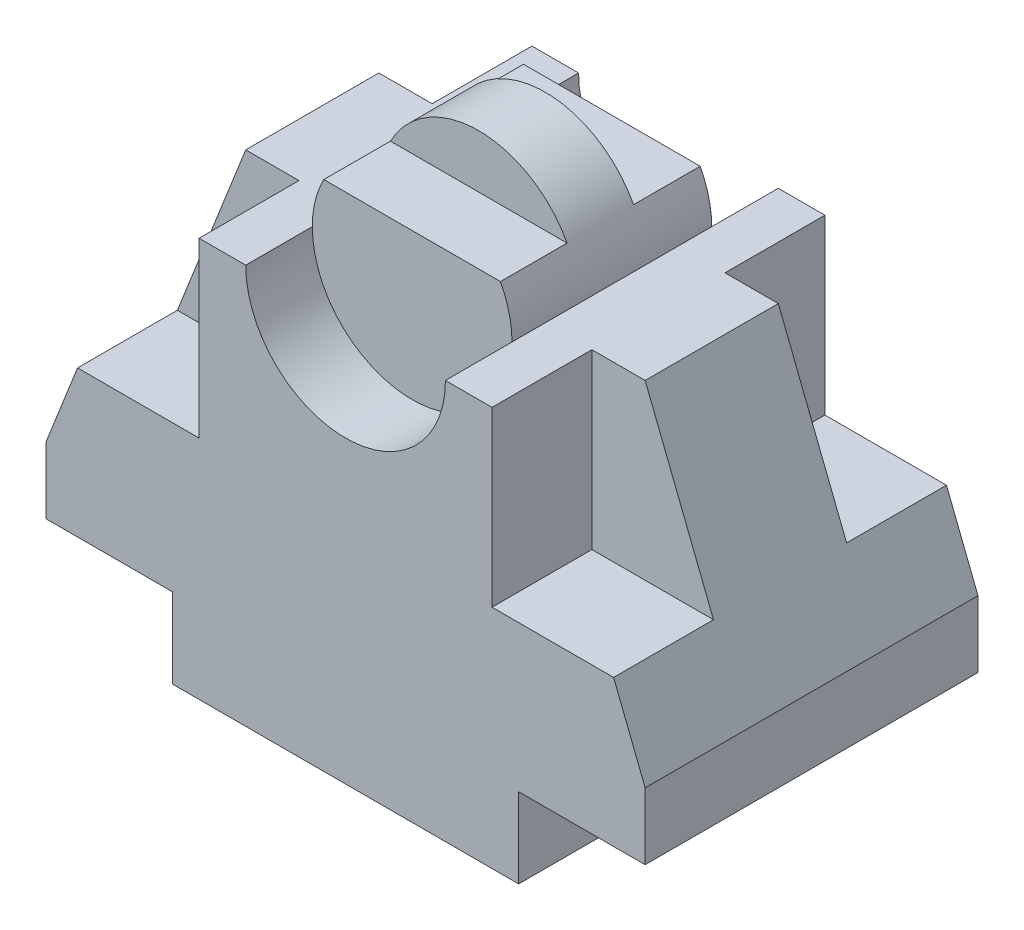
ISO-10303-21;
HEADER;
FILE_DESCRIPTION(('STEP AP214'),'2;1');
FILE_NAME('part.step','',(''),(''),'','','');
FILE_SCHEMA(('AUTOMOTIVE_DESIGN { 1 0 10303 214 1 1 1 1 }'));
ENDSEC;
DATA;
#1=APPLICATION_CONTEXT('core data for automotive mechanical design processes');
#2=APPLICATION_PROTOCOL_DEFINITION('international standard','automotive_design',2000,#1);
#3=PRODUCT_CONTEXT('',#1,'mechanical');
#4=PRODUCT('Part','Part','',(#3));
#5=PRODUCT_RELATED_PRODUCT_CATEGORY('part','',(#4));
#6=PRODUCT_DEFINITION_FORMATION('','',#4);
#7=PRODUCT_DEFINITION_CONTEXT('part definition',#1,'design');
#8=PRODUCT_DEFINITION('design','',#6,#7);
#9=PRODUCT_DEFINITION_SHAPE('','',#8);
#10=(LENGTH_UNIT() NAMED_UNIT(*) SI_UNIT(.MILLI.,.METRE.));
#11=(NAMED_UNIT(*) PLANE_ANGLE_UNIT() SI_UNIT($,.RADIAN.));
#12=(NAMED_UNIT(*) SI_UNIT($,.STERADIAN.) SOLID_ANGLE_UNIT());
#13=UNCERTAINTY_MEASURE_WITH_UNIT(LENGTH_MEASURE(1.E-05),#10,'distance_accuracy_value','');
#14=(GEOMETRIC_REPRESENTATION_CONTEXT(3) GLOBAL_UNCERTAINTY_ASSIGNED_CONTEXT((#13)) GLOBAL_UNIT_ASSIGNED_CONTEXT((#10,
#11,#12)) REPRESENTATION_CONTEXT('',''));
#15=CARTESIAN_POINT('',(0.,0.,0.));
#16=DIRECTION('',(0.,0.,1.));
#17=DIRECTION('',(1.,0.,0.));
#18=AXIS2_PLACEMENT_3D('',#15,#16,#17);
#19=CARTESIAN_POINT('',(0.,48.,15.));
#20=DIRECTION('',(0.,0.,-1.));
#21=DIRECTION('',(-1.,0.,0.));
#22=AXIS2_PLACEMENT_3D('',#19,#20,#21);
#23=CYLINDRICAL_SURFACE('',#22,15.);
#24=DIRECTION('',(0.,0.,-1.));
#25=VECTOR('',#24,1.);
#26=CARTESIAN_POINT('',(13.2664991614216,55.,15.));
#27=LINE('',#26,#25);
#28=CARTESIAN_POINT('',(13.2664991614216,55.,15.));
#29=VERTEX_POINT('',#28);
#30=CARTESIAN_POINT('',(13.2664991614216,55.,5.));
#31=VERTEX_POINT('',#30);
#32=EDGE_CURVE('E239',#29,#31,#27,.T.);
#33=ORIENTED_EDGE('',*,*,#32,.F.);
#34=CARTESIAN_POINT('',(0.,48.,15.));
#35=DIRECTION('',(0.,0.,1.));
#36=DIRECTION('',(1.,0.,0.));
#37=AXIS2_PLACEMENT_3D('',#34,#35,#36);
#38=CIRCLE('',#37,15.);
#39=CARTESIAN_POINT('',(15.,48.,15.));
#40=VERTEX_POINT('',#39);
#41=EDGE_CURVE('E249',#40,#29,#38,.T.);
#42=ORIENTED_EDGE('',*,*,#41,.F.);
#43=DIRECTION('',(0.,0.,1.));
#44=VECTOR('',#43,1.);
#45=CARTESIAN_POINT('',(15.,48.,-25.));
#46=LINE('',#45,#44);
#47=CARTESIAN_POINT('',(15.,48.,-15.));
#48=VERTEX_POINT('',#47);
#49=EDGE_CURVE('E275',#40,#48,#46,.F.);
#50=ORIENTED_EDGE('',*,*,#49,.T.);
#51=CARTESIAN_POINT('',(0.,48.,-15.));
#52=DIRECTION('',(0.,0.,1.));
#53=DIRECTION('',(1.,0.,0.));
#54=AXIS2_PLACEMENT_3D('',#51,#52,#53);
#55=CIRCLE('',#54,15.);
#56=CARTESIAN_POINT('',(13.2664991614216,55.,-15.));
#57=VERTEX_POINT('',#56);
#58=EDGE_CURVE('E257',#48,#57,#55,.T.);
#59=ORIENTED_EDGE('',*,*,#58,.T.);
#60=DIRECTION('',(0.,0.,-1.));
#61=VECTOR('',#60,1.);
#62=CARTESIAN_POINT('',(13.2664991614216,55.,15.));
#63=LINE('',#62,#61);
#64=CARTESIAN_POINT('',(13.2664991614216,55.,-5.));
#65=VERTEX_POINT('',#64);
#66=EDGE_CURVE('E62',#57,#65,#63,.F.);
#67=ORIENTED_EDGE('',*,*,#66,.T.);
#68=CARTESIAN_POINT('',(0.,48.,-5.));
#69=DIRECTION('',(0.,0.,1.));
#70=DIRECTION('',(1.,0.,0.));
#71=AXIS2_PLACEMENT_3D('',#68,#69,#70);
#72=CIRCLE('',#71,15.);
#73=CARTESIAN_POINT('',(-13.2664991614216,55.,-5.));
#74=VERTEX_POINT('',#73);
#75=EDGE_CURVE('E242',#65,#74,#72,.T.);
#76=ORIENTED_EDGE('',*,*,#75,.T.);
#77=DIRECTION('',(0.,0.,-1.));
#78=VECTOR('',#77,1.);
#79=CARTESIAN_POINT('',(-13.2664991614216,55.,15.));
#80=LINE('',#79,#78);
#81=CARTESIAN_POINT('',(-13.2664991614216,55.,-15.));
#82=VERTEX_POINT('',#81);
#83=EDGE_CURVE('E263',#74,#82,#80,.T.);
#84=ORIENTED_EDGE('',*,*,#83,.T.);
#85=CARTESIAN_POINT('',(-15.,48.,-15.));
#86=VERTEX_POINT('',#85);
#87=EDGE_CURVE('E266',#82,#86,#55,.T.);
#88=ORIENTED_EDGE('',*,*,#87,.T.);
#89=DIRECTION('',(0.,0.,1.));
#90=VECTOR('',#89,1.);
#91=CARTESIAN_POINT('',(-15.,48.,-25.));
#92=LINE('',#91,#90);
#93=CARTESIAN_POINT('',(-15.,48.,15.));
#94=VERTEX_POINT('',#93);
#95=EDGE_CURVE('E280',#86,#94,#92,.T.);
#96=ORIENTED_EDGE('',*,*,#95,.T.);
#97=CARTESIAN_POINT('',(-13.2664991614216,55.,15.));
#98=VERTEX_POINT('',#97);
#99=EDGE_CURVE('E258',#98,#94,#38,.T.);
#100=ORIENTED_EDGE('',*,*,#99,.F.);
#101=DIRECTION('',(0.,0.,-1.));
#102=VECTOR('',#101,1.);
#103=CARTESIAN_POINT('',(-13.2664991614216,55.,15.));
#104=LINE('',#103,#102);
#105=CARTESIAN_POINT('',(-13.2664991614216,55.,5.));
#106=VERTEX_POINT('',#105);
#107=EDGE_CURVE('E57',#106,#98,#104,.F.);
#108=ORIENTED_EDGE('',*,*,#107,.F.);
#109=CARTESIAN_POINT('',(0.,48.,5.));
#110=DIRECTION('',(0.,0.,1.));
#111=DIRECTION('',(1.,0.,0.));
#112=AXIS2_PLACEMENT_3D('',#109,#110,#111);
#113=CIRCLE('',#112,15.);
#114=EDGE_CURVE('E11',#31,#106,#113,.T.);
#115=ORIENTED_EDGE('',*,*,#114,.F.);
#116=EDGE_LOOP('',(#33,#42,#50,#59,#67,#76,#84,#88,#96,#100,#108,#115));
#117=FACE_BOUND('',#116,.T.);
#118=ADVANCED_FACE('F41',(#117),#23,.T.);
#119=CARTESIAN_POINT('',(0.,48.,15.));
#120=DIRECTION('',(0.,0.,1.));
#121=DIRECTION('',(1.,0.,0.));
#122=AXIS2_PLACEMENT_3D('',#119,#120,#121);
#123=PLANE('',#122);
#124=ORIENTED_EDGE('',*,*,#41,.T.);
#125=DIRECTION('',(-1.,0.,0.));
#126=VECTOR('',#125,1.);
#127=CARTESIAN_POINT('',(0.,55.,15.));
#128=LINE('',#127,#126);
#129=EDGE_CURVE('E47',#29,#98,#128,.T.);
#130=ORIENTED_EDGE('',*,*,#129,.T.);
#131=ORIENTED_EDGE('',*,*,#99,.T.);
#132=CARTESIAN_POINT('',(0.,48.,15.));
#133=DIRECTION('',(0.,0.,1.));
#134=DIRECTION('',(1.,0.,0.));
#135=AXIS2_PLACEMENT_3D('',#132,#133,#134);
#136=CIRCLE('',#135,15.);
#137=EDGE_CURVE('E255',#40,#94,#136,.F.);
#138=ORIENTED_EDGE('',*,*,#137,.F.);
#139=EDGE_LOOP('',(#124,#130,#131,#138));
#140=FACE_BOUND('',#139,.T.);
#141=ADVANCED_FACE('F252',(#140),#123,.T.);
#142=CARTESIAN_POINT('',(0.,48.,-25.));
#143=DIRECTION('',(0.,0.,1.));
#144=DIRECTION('',(1.,0.,0.));
#145=AXIS2_PLACEMENT_3D('',#142,#143,#144);
#146=CYLINDRICAL_SURFACE('',#145,15.);
#147=CARTESIAN_POINT('',(0.,48.,-15.));
#148=DIRECTION('',(0.,0.,1.));
#149=DIRECTION('',(1.,0.,0.));
#150=AXIS2_PLACEMENT_3D('',#147,#148,#149);
#151=CIRCLE('',#150,15.);
#152=EDGE_CURVE('E457',#48,#86,#151,.F.);
#153=ORIENTED_EDGE('',*,*,#152,.F.);
#154=CARTESIAN_POINT('',(15.,48.,-25.));
#155=VERTEX_POINT('',#154);
#156=EDGE_CURVE('E256',#48,#155,#46,.F.);
#157=ORIENTED_EDGE('',*,*,#156,.T.);
#158=CARTESIAN_POINT('',(0.,48.,-25.));
#159=DIRECTION('',(0.,0.,1.));
#160=DIRECTION('',(1.,0.,0.));
#161=AXIS2_PLACEMENT_3D('',#158,#159,#160);
#162=CIRCLE('',#161,15.);
#163=CARTESIAN_POINT('',(-15.,48.,-25.));
#164=VERTEX_POINT('',#163);
#165=EDGE_CURVE('E454',#164,#155,#162,.T.);
#166=ORIENTED_EDGE('',*,*,#165,.F.);
#167=EDGE_CURVE('E272',#164,#86,#92,.T.);
#168=ORIENTED_EDGE('',*,*,#167,.T.);
#169=EDGE_LOOP('',(#153,#157,#166,#168));
#170=FACE_BOUND('',#169,.T.);
#171=ADVANCED_FACE('F499',(#170),#146,.F.);
#172=CARTESIAN_POINT('',(0.,48.,25.));
#173=DIRECTION('',(0.,1.,0.));
#174=DIRECTION('',(0.,0.,1.));
#175=AXIS2_PLACEMENT_3D('',#172,#173,#174);
#176=PLANE('',#175);
#177=ORIENTED_EDGE('',*,*,#167,.F.);
#178=DIRECTION('',(1.,0.,0.));
#179=VECTOR('',#178,1.);
#180=CARTESIAN_POINT('',(0.,48.,-25.));
#181=LINE('',#180,#179);
#182=CARTESIAN_POINT('',(-22.,48.,-25.));
#183=VERTEX_POINT('',#182);
#184=EDGE_CURVE('E405',#183,#164,#181,.T.);
#185=ORIENTED_EDGE('',*,*,#184,.F.);
#186=DIRECTION('',(0.,0.,-1.));
#187=VECTOR('',#186,1.);
#188=CARTESIAN_POINT('',(-22.,48.,-10.));
#189=LINE('',#188,#187);
#190=CARTESIAN_POINT('',(-22.,48.,-10.));
#191=VERTEX_POINT('',#190);
#192=EDGE_CURVE('E340',#191,#183,#189,.T.);
#193=ORIENTED_EDGE('',*,*,#192,.F.);
#194=DIRECTION('',(-1.,0.,0.));
#195=VECTOR('',#194,1.);
#196=CARTESIAN_POINT('',(-30.,48.,-10.));
#197=LINE('',#196,#195);
#198=CARTESIAN_POINT('',(-30.,48.,-10.));
#199=VERTEX_POINT('',#198);
#200=EDGE_CURVE('E328',#191,#199,#197,.T.);
#201=ORIENTED_EDGE('',*,*,#200,.T.);
#202=DIRECTION('',(0.,0.,-1.));
#203=VECTOR('',#202,1.);
#204=CARTESIAN_POINT('',(-30.,48.,25.));
#205=LINE('',#204,#203);
#206=CARTESIAN_POINT('',(-30.,48.,10.));
#207=VERTEX_POINT('',#206);
#208=EDGE_CURVE('E449',#207,#199,#205,.T.);
#209=ORIENTED_EDGE('',*,*,#208,.F.);
#210=DIRECTION('',(-1.,0.,0.));
#211=VECTOR('',#210,1.);
#212=CARTESIAN_POINT('',(-30.,48.,10.));
#213=LINE('',#212,#211);
#214=CARTESIAN_POINT('',(-22.,48.,10.));
#215=VERTEX_POINT('',#214);
#216=EDGE_CURVE('E356',#215,#207,#213,.T.);
#217=ORIENTED_EDGE('',*,*,#216,.F.);
#218=DIRECTION('',(0.,0.,1.));
#219=VECTOR('',#218,1.);
#220=CARTESIAN_POINT('',(-22.,48.,10.));
#221=LINE('',#220,#219);
#222=CARTESIAN_POINT('',(-22.,48.,25.));
#223=VERTEX_POINT('',#222);
#224=EDGE_CURVE('E364',#215,#223,#221,.T.);
#225=ORIENTED_EDGE('',*,*,#224,.T.);
#226=DIRECTION('',(1.,0.,0.));
#227=VECTOR('',#226,1.);
#228=CARTESIAN_POINT('',(0.,48.,25.));
#229=LINE('',#228,#227);
#230=CARTESIAN_POINT('',(-15.,48.,25.));
#231=VERTEX_POINT('',#230);
#232=EDGE_CURVE('E375',#223,#231,#229,.T.);
#233=ORIENTED_EDGE('',*,*,#232,.T.);
#234=EDGE_CURVE('E271',#94,#231,#92,.T.);
#235=ORIENTED_EDGE('',*,*,#234,.F.);
#236=ORIENTED_EDGE('',*,*,#95,.F.);
#237=EDGE_LOOP('',(#177,#185,#193,#201,#209,#217,#225,#233,#235,#236));
#238=FACE_BOUND('',#237,.T.);
#239=ADVANCED_FACE('F482',(#238),#176,.T.);
#240=CARTESIAN_POINT('',(15.,48.,25.));
#241=VERTEX_POINT('',#240);
#242=EDGE_CURVE('E268',#241,#40,#46,.F.);
#243=ORIENTED_EDGE('',*,*,#242,.F.);
#244=CARTESIAN_POINT('',(22.,48.,25.));
#245=VERTEX_POINT('',#244);
#246=EDGE_CURVE('E376',#241,#245,#229,.T.);
#247=ORIENTED_EDGE('',*,*,#246,.T.);
#248=DIRECTION('',(0.,0.,1.));
#249=VECTOR('',#248,1.);
#250=CARTESIAN_POINT('',(22.,48.,10.));
#251=LINE('',#250,#249);
#252=CARTESIAN_POINT('',(22.,48.,10.));
#253=VERTEX_POINT('',#252);
#254=EDGE_CURVE('E311',#253,#245,#251,.T.);
#255=ORIENTED_EDGE('',*,*,#254,.F.);
#256=DIRECTION('',(1.,0.,0.));
#257=VECTOR('',#256,1.);
#258=CARTESIAN_POINT('',(30.,48.,10.));
#259=LINE('',#258,#257);
#260=CARTESIAN_POINT('',(30.,48.,10.));
#261=VERTEX_POINT('',#260);
#262=EDGE_CURVE('E303',#253,#261,#259,.T.);
#263=ORIENTED_EDGE('',*,*,#262,.T.);
#264=DIRECTION('',(0.,0.,-1.));
#265=VECTOR('',#264,1.);
#266=CARTESIAN_POINT('',(30.,48.,25.));
#267=LINE('',#266,#265);
#268=CARTESIAN_POINT('',(30.,48.,-10.));
#269=VERTEX_POINT('',#268);
#270=EDGE_CURVE('E402',#261,#269,#267,.T.);
#271=ORIENTED_EDGE('',*,*,#270,.T.);
#272=DIRECTION('',(1.,0.,0.));
#273=VECTOR('',#272,1.);
#274=CARTESIAN_POINT('',(30.,48.,-10.));
#275=LINE('',#274,#273);
#276=CARTESIAN_POINT('',(22.,48.,-10.));
#277=VERTEX_POINT('',#276);
#278=EDGE_CURVE('E289',#277,#269,#275,.T.);
#279=ORIENTED_EDGE('',*,*,#278,.F.);
#280=DIRECTION('',(0.,0.,-1.));
#281=VECTOR('',#280,1.);
#282=CARTESIAN_POINT('',(22.,48.,-10.));
#283=LINE('',#282,#281);
#284=CARTESIAN_POINT('',(22.,48.,-25.));
#285=VERTEX_POINT('',#284);
#286=EDGE_CURVE('E293',#277,#285,#283,.T.);
#287=ORIENTED_EDGE('',*,*,#286,.T.);
#288=EDGE_CURVE('E366',#155,#285,#181,.T.);
#289=ORIENTED_EDGE('',*,*,#288,.F.);
#290=ORIENTED_EDGE('',*,*,#156,.F.);
#291=ORIENTED_EDGE('',*,*,#49,.F.);
#292=EDGE_LOOP('',(#243,#247,#255,#263,#271,#279,#287,#289,#290,#291));
#293=FACE_BOUND('',#292,.T.);
#294=ADVANCED_FACE('F43',(#293),#176,.T.);
#295=CARTESIAN_POINT('',(42.3487118034751,16.7165967645297,25.));
#296=DIRECTION('',(0.930155221331323,0.367166534736049,0.));
#297=DIRECTION('',(-0.367166534736049,0.930155221331323,0.));
#298=AXIS2_PLACEMENT_3D('',#295,#296,#297);
#299=PLANE('',#298);
#300=DIRECTION('',(0.,0.,-1.));
#301=VECTOR('',#300,1.);
#302=CARTESIAN_POINT('',(40.2631578947368,22.,-10.));
#303=LINE('',#302,#301);
#304=CARTESIAN_POINT('',(40.2631578947368,22.,-10.));
#305=VERTEX_POINT('',#304);
#306=CARTESIAN_POINT('',(40.2631578947368,22.,-25.));
#307=VERTEX_POINT('',#306);
#308=EDGE_CURVE('E288',#305,#307,#303,.T.);
#309=ORIENTED_EDGE('',*,*,#308,.F.);
#310=DIRECTION('',(0.367166534736048,-0.930155221331323,0.));
#311=VECTOR('',#310,1.);
#312=CARTESIAN_POINT('',(40.2631578947368,22.,-10.));
#313=LINE('',#312,#311);
#314=EDGE_CURVE('E279',#269,#305,#313,.T.);
#315=ORIENTED_EDGE('',*,*,#314,.F.);
#316=ORIENTED_EDGE('',*,*,#270,.F.);
#317=DIRECTION('',(0.367166534736048,-0.930155221331323,0.));
#318=VECTOR('',#317,1.);
#319=CARTESIAN_POINT('',(40.2631578947368,22.,10.));
#320=LINE('',#319,#318);
#321=CARTESIAN_POINT('',(40.2631578947368,22.,10.));
#322=VERTEX_POINT('',#321);
#323=EDGE_CURVE('E305',#261,#322,#320,.T.);
#324=ORIENTED_EDGE('',*,*,#323,.T.);
#325=DIRECTION('',(0.,0.,1.));
#326=VECTOR('',#325,1.);
#327=CARTESIAN_POINT('',(40.2631578947368,22.,10.));
#328=LINE('',#327,#326);
#329=CARTESIAN_POINT('',(40.2631578947368,22.,25.));
#330=VERTEX_POINT('',#329);
#331=EDGE_CURVE('E318',#322,#330,#328,.T.);
#332=ORIENTED_EDGE('',*,*,#331,.T.);
#333=DIRECTION('',(0.367166534736048,-0.930155221331323,0.));
#334=VECTOR('',#333,1.);
#335=CARTESIAN_POINT('',(42.3487118034751,16.7165967645297,25.));
#336=LINE('',#335,#334);
#337=CARTESIAN_POINT('',(45.,10.,25.));
#338=VERTEX_POINT('',#337);
#339=EDGE_CURVE('E396',#330,#338,#336,.T.);
#340=ORIENTED_EDGE('',*,*,#339,.T.);
#341=DIRECTION('',(0.,0.,-1.));
#342=VECTOR('',#341,1.);
#343=CARTESIAN_POINT('',(45.,10.,25.));
#344=LINE('',#343,#342);
#345=CARTESIAN_POINT('',(45.,10.,-25.));
#346=VERTEX_POINT('',#345);
#347=EDGE_CURVE('E433',#338,#346,#344,.T.);
#348=ORIENTED_EDGE('',*,*,#347,.T.);
#349=DIRECTION('',(0.367166534736048,-0.930155221331323,0.));
#350=VECTOR('',#349,1.);
#351=CARTESIAN_POINT('',(42.3487118034751,16.7165967645297,-25.));
#352=LINE('',#351,#350);
#353=EDGE_CURVE('E427',#307,#346,#352,.T.);
#354=ORIENTED_EDGE('',*,*,#353,.F.);
#355=EDGE_LOOP('',(#309,#315,#316,#324,#332,#340,#348,#354));
#356=FACE_BOUND('',#355,.T.);
#357=ADVANCED_FACE('F518',(#356),#299,.T.);
#358=CARTESIAN_POINT('',(0.,0.,25.));
#359=DIRECTION('',(0.,0.,1.));
#360=DIRECTION('',(1.,0.,0.));
#361=AXIS2_PLACEMENT_3D('',#358,#359,#360);
#362=PLANE('',#361);
#363=CARTESIAN_POINT('',(0.,48.,25.));
#364=DIRECTION('',(0.,0.,1.));
#365=DIRECTION('',(1.,0.,0.));
#366=AXIS2_PLACEMENT_3D('',#363,#364,#365);
#367=CIRCLE('',#366,15.);
#368=EDGE_CURVE('E254',#231,#241,#367,.T.);
#369=ORIENTED_EDGE('',*,*,#368,.F.);
#370=ORIENTED_EDGE('',*,*,#232,.F.);
#371=DIRECTION('',(0.,1.,0.));
#372=VECTOR('',#371,1.);
#373=CARTESIAN_POINT('',(-22.,48.,25.));
#374=LINE('',#373,#372);
#375=CARTESIAN_POINT('',(-22.,22.,25.));
#376=VERTEX_POINT('',#375);
#377=EDGE_CURVE('E351',#376,#223,#374,.T.);
#378=ORIENTED_EDGE('',*,*,#377,.F.);
#379=DIRECTION('',(1.,0.,0.));
#380=VECTOR('',#379,1.);
#381=CARTESIAN_POINT('',(-22.,22.,25.));
#382=LINE('',#381,#380);
#383=CARTESIAN_POINT('',(-40.2631578947368,22.,25.));
#384=VERTEX_POINT('',#383);
#385=EDGE_CURVE('E343',#384,#376,#382,.T.);
#386=ORIENTED_EDGE('',*,*,#385,.F.);
#387=DIRECTION('',(0.367166534736048,0.930155221331323,0.));
#388=VECTOR('',#387,1.);
#389=CARTESIAN_POINT('',(-42.3487118034751,16.7165967645297,25.));
#390=LINE('',#389,#388);
#391=CARTESIAN_POINT('',(-45.,10.,25.));
#392=VERTEX_POINT('',#391);
#393=EDGE_CURVE('E374',#392,#384,#390,.T.);
#394=ORIENTED_EDGE('',*,*,#393,.F.);
#395=DIRECTION('',(0.,1.,0.));
#396=VECTOR('',#395,1.);
#397=CARTESIAN_POINT('',(-45.,0.,25.));
#398=LINE('',#397,#396);
#399=CARTESIAN_POINT('',(-45.,0.,25.));
#400=VERTEX_POINT('',#399);
#401=EDGE_CURVE('E377',#400,#392,#398,.T.);
#402=ORIENTED_EDGE('',*,*,#401,.F.);
#403=DIRECTION('',(-1.,0.,0.));
#404=VECTOR('',#403,1.);
#405=CARTESIAN_POINT('',(0.,0.,25.));
#406=LINE('',#405,#404);
#407=CARTESIAN_POINT('',(-26.,0.,25.));
#408=VERTEX_POINT('',#407);
#409=EDGE_CURVE('E385',#408,#400,#406,.T.);
#410=ORIENTED_EDGE('',*,*,#409,.F.);
#411=DIRECTION('',(0.,1.,0.));
#412=VECTOR('',#411,1.);
#413=CARTESIAN_POINT('',(-26.,0.,25.));
#414=LINE('',#413,#412);
#415=CARTESIAN_POINT('',(-26.,-12.,25.));
#416=VERTEX_POINT('',#415);
#417=EDGE_CURVE('E384',#416,#408,#414,.T.);
#418=ORIENTED_EDGE('',*,*,#417,.F.);
#419=DIRECTION('',(-1.,0.,0.));
#420=VECTOR('',#419,1.);
#421=CARTESIAN_POINT('',(0.,-12.,25.));
#422=LINE('',#421,#420);
#423=CARTESIAN_POINT('',(26.,-12.,25.));
#424=VERTEX_POINT('',#423);
#425=EDGE_CURVE('E389',#424,#416,#422,.T.);
#426=ORIENTED_EDGE('',*,*,#425,.F.);
#427=DIRECTION('',(0.,-1.,0.));
#428=VECTOR('',#427,1.);
#429=CARTESIAN_POINT('',(26.,0.,25.));
#430=LINE('',#429,#428);
#431=CARTESIAN_POINT('',(26.,0.,25.));
#432=VERTEX_POINT('',#431);
#433=EDGE_CURVE('E393',#432,#424,#430,.T.);
#434=ORIENTED_EDGE('',*,*,#433,.F.);
#435=DIRECTION('',(1.,0.,0.));
#436=VECTOR('',#435,1.);
#437=CARTESIAN_POINT('',(0.,0.,25.));
#438=LINE('',#437,#436);
#439=CARTESIAN_POINT('',(45.,0.,25.));
#440=VERTEX_POINT('',#439);
#441=EDGE_CURVE('E392',#432,#440,#438,.T.);
#442=ORIENTED_EDGE('',*,*,#441,.T.);
#443=DIRECTION('',(0.,-1.,0.));
#444=VECTOR('',#443,1.);
#445=CARTESIAN_POINT('',(45.,0.,25.));
#446=LINE('',#445,#444);
#447=EDGE_CURVE('E397',#338,#440,#446,.T.);
#448=ORIENTED_EDGE('',*,*,#447,.F.);
#449=ORIENTED_EDGE('',*,*,#339,.F.);
#450=DIRECTION('',(-1.,0.,0.));
#451=VECTOR('',#450,1.);
#452=CARTESIAN_POINT('',(22.,22.,25.));
#453=LINE('',#452,#451);
#454=CARTESIAN_POINT('',(22.,22.,25.));
#455=VERTEX_POINT('',#454);
#456=EDGE_CURVE('E308',#330,#455,#453,.T.);
#457=ORIENTED_EDGE('',*,*,#456,.T.);
#458=DIRECTION('',(0.,1.,0.));
#459=VECTOR('',#458,1.);
#460=CARTESIAN_POINT('',(22.,48.,25.));
#461=LINE('',#460,#459);
#462=EDGE_CURVE('E296',#455,#245,#461,.T.);
#463=ORIENTED_EDGE('',*,*,#462,.T.);
#464=ORIENTED_EDGE('',*,*,#246,.F.);
#465=EDGE_LOOP('',(#369,#370,#378,#386,#394,#402,#410,#418,#426,#434,#442,#448,#449,#457,#463,#464));
#466=FACE_BOUND('',#465,.T.);
#467=ADVANCED_FACE('F487',(#466),#362,.T.);
#468=CARTESIAN_POINT('',(-42.3487118034751,16.7165967645297,25.));
#469=DIRECTION('',(-0.930155221331323,0.367166534736049,0.));
#470=DIRECTION('',(-0.367166534736049,-0.930155221331323,0.));
#471=AXIS2_PLACEMENT_3D('',#468,#469,#470);
#472=PLANE('',#471);
#473=DIRECTION('',(-0.367166534736048,-0.930155221331323,0.));
#474=VECTOR('',#473,1.);
#475=CARTESIAN_POINT('',(-40.2631578947368,22.,-10.));
#476=LINE('',#475,#474);
#477=CARTESIAN_POINT('',(-40.2631578947368,22.,-10.));
#478=VERTEX_POINT('',#477);
#479=EDGE_CURVE('E326',#199,#478,#476,.T.);
#480=ORIENTED_EDGE('',*,*,#479,.T.);
#481=DIRECTION('',(0.,0.,-1.));
#482=VECTOR('',#481,1.);
#483=CARTESIAN_POINT('',(-40.2631578947368,22.,-10.));
#484=LINE('',#483,#482);
#485=CARTESIAN_POINT('',(-40.2631578947368,22.,-25.));
#486=VERTEX_POINT('',#485);
#487=EDGE_CURVE('E345',#478,#486,#484,.T.);
#488=ORIENTED_EDGE('',*,*,#487,.T.);
#489=DIRECTION('',(0.367166534736048,0.930155221331323,0.));
#490=VECTOR('',#489,1.);
#491=CARTESIAN_POINT('',(-42.3487118034751,16.7165967645297,-25.));
#492=LINE('',#491,#490);
#493=CARTESIAN_POINT('',(-45.,10.,-25.));
#494=VERTEX_POINT('',#493);
#495=EDGE_CURVE('E403',#494,#486,#492,.T.);
#496=ORIENTED_EDGE('',*,*,#495,.F.);
#497=DIRECTION('',(0.,0.,-1.));
#498=VECTOR('',#497,1.);
#499=CARTESIAN_POINT('',(-45.,10.,25.));
#500=LINE('',#499,#498);
#501=EDGE_CURVE('E446',#392,#494,#500,.T.);
#502=ORIENTED_EDGE('',*,*,#501,.F.);
#503=ORIENTED_EDGE('',*,*,#393,.T.);
#504=DIRECTION('',(0.,0.,1.));
#505=VECTOR('',#504,1.);
#506=CARTESIAN_POINT('',(-40.2631578947368,22.,10.));
#507=LINE('',#506,#505);
#508=CARTESIAN_POINT('',(-40.2631578947368,22.,10.));
#509=VERTEX_POINT('',#508);
#510=EDGE_CURVE('E363',#509,#384,#507,.T.);
#511=ORIENTED_EDGE('',*,*,#510,.F.);
#512=DIRECTION('',(-0.367166534736048,-0.930155221331323,0.));
#513=VECTOR('',#512,1.);
#514=CARTESIAN_POINT('',(-40.2631578947368,22.,10.));
#515=LINE('',#514,#513);
#516=EDGE_CURVE('E349',#207,#509,#515,.T.);
#517=ORIENTED_EDGE('',*,*,#516,.F.);
#518=ORIENTED_EDGE('',*,*,#208,.T.);
#519=EDGE_LOOP('',(#480,#488,#496,#502,#503,#511,#517,#518));
#520=FACE_BOUND('',#519,.T.);
#521=ADVANCED_FACE('F548',(#520),#472,.T.);
#522=CARTESIAN_POINT('',(0.,0.,-25.));
#523=DIRECTION('',(0.,0.,1.));
#524=DIRECTION('',(1.,0.,0.));
#525=AXIS2_PLACEMENT_3D('',#522,#523,#524);
#526=PLANE('',#525);
#527=ORIENTED_EDGE('',*,*,#184,.T.);
#528=ORIENTED_EDGE('',*,*,#165,.T.);
#529=ORIENTED_EDGE('',*,*,#288,.T.);
#530=DIRECTION('',(0.,1.,0.));
#531=VECTOR('',#530,1.);
#532=CARTESIAN_POINT('',(22.,48.,-25.));
#533=LINE('',#532,#531);
#534=CARTESIAN_POINT('',(22.,22.,-25.));
#535=VERTEX_POINT('',#534);
#536=EDGE_CURVE('E285',#535,#285,#533,.T.);
#537=ORIENTED_EDGE('',*,*,#536,.F.);
#538=DIRECTION('',(-1.,0.,0.));
#539=VECTOR('',#538,1.);
#540=CARTESIAN_POINT('',(22.,22.,-25.));
#541=LINE('',#540,#539);
#542=EDGE_CURVE('E277',#307,#535,#541,.T.);
#543=ORIENTED_EDGE('',*,*,#542,.F.);
#544=ORIENTED_EDGE('',*,*,#353,.T.);
#545=DIRECTION('',(0.,-1.,0.));
#546=VECTOR('',#545,1.);
#547=CARTESIAN_POINT('',(45.,0.,-25.));
#548=LINE('',#547,#546);
#549=CARTESIAN_POINT('',(45.,0.,-25.));
#550=VERTEX_POINT('',#549);
#551=EDGE_CURVE('E426',#346,#550,#548,.T.);
#552=ORIENTED_EDGE('',*,*,#551,.T.);
#553=DIRECTION('',(1.,0.,0.));
#554=VECTOR('',#553,1.);
#555=CARTESIAN_POINT('',(0.,0.,-25.));
#556=LINE('',#555,#554);
#557=CARTESIAN_POINT('',(26.,0.,-25.));
#558=VERTEX_POINT('',#557);
#559=EDGE_CURVE('E421',#558,#550,#556,.T.);
#560=ORIENTED_EDGE('',*,*,#559,.F.);
#561=DIRECTION('',(0.,-1.,0.));
#562=VECTOR('',#561,1.);
#563=CARTESIAN_POINT('',(26.,0.,-25.));
#564=LINE('',#563,#562);
#565=CARTESIAN_POINT('',(26.,-12.,-25.));
#566=VERTEX_POINT('',#565);
#567=EDGE_CURVE('E419',#558,#566,#564,.T.);
#568=ORIENTED_EDGE('',*,*,#567,.T.);
#569=DIRECTION('',(-1.,0.,0.));
#570=VECTOR('',#569,1.);
#571=CARTESIAN_POINT('',(0.,-12.,-25.));
#572=LINE('',#571,#570);
#573=CARTESIAN_POINT('',(-26.,-12.,-25.));
#574=VERTEX_POINT('',#573);
#575=EDGE_CURVE('E417',#566,#574,#572,.T.);
#576=ORIENTED_EDGE('',*,*,#575,.T.);
#577=DIRECTION('',(0.,1.,0.));
#578=VECTOR('',#577,1.);
#579=CARTESIAN_POINT('',(-26.,0.,-25.));
#580=LINE('',#579,#578);
#581=CARTESIAN_POINT('',(-26.,0.,-25.));
#582=VERTEX_POINT('',#581);
#583=EDGE_CURVE('E411',#574,#582,#580,.T.);
#584=ORIENTED_EDGE('',*,*,#583,.T.);
#585=DIRECTION('',(-1.,0.,0.));
#586=VECTOR('',#585,1.);
#587=CARTESIAN_POINT('',(0.,0.,-25.));
#588=LINE('',#587,#586);
#589=CARTESIAN_POINT('',(-45.,0.,-25.));
#590=VERTEX_POINT('',#589);
#591=EDGE_CURVE('E412',#582,#590,#588,.T.);
#592=ORIENTED_EDGE('',*,*,#591,.T.);
#593=DIRECTION('',(0.,1.,0.));
#594=VECTOR('',#593,1.);
#595=CARTESIAN_POINT('',(-45.,0.,-25.));
#596=LINE('',#595,#594);
#597=EDGE_CURVE('E406',#590,#494,#596,.T.);
#598=ORIENTED_EDGE('',*,*,#597,.T.);
#599=ORIENTED_EDGE('',*,*,#495,.T.);
#600=DIRECTION('',(1.,0.,0.));
#601=VECTOR('',#600,1.);
#602=CARTESIAN_POINT('',(-22.,22.,-25.));
#603=LINE('',#602,#601);
#604=CARTESIAN_POINT('',(-22.,22.,-25.));
#605=VERTEX_POINT('',#604);
#606=EDGE_CURVE('E329',#486,#605,#603,.T.);
#607=ORIENTED_EDGE('',*,*,#606,.T.);
#608=DIRECTION('',(0.,1.,0.));
#609=VECTOR('',#608,1.);
#610=CARTESIAN_POINT('',(-22.,48.,-25.));
#611=LINE('',#610,#609);
#612=EDGE_CURVE('E321',#605,#183,#611,.T.);
#613=ORIENTED_EDGE('',*,*,#612,.T.);
#614=EDGE_LOOP('',(#527,#528,#529,#537,#543,#544,#552,#560,#568,#576,#584,#592,#598,#599,#607,#613));
#615=FACE_BOUND('',#614,.T.);
#616=ADVANCED_FACE('F498',(#615),#526,.F.);
#617=CARTESIAN_POINT('',(-45.,0.,25.));
#618=DIRECTION('',(-1.,0.,0.));
#619=DIRECTION('',(0.,0.,1.));
#620=AXIS2_PLACEMENT_3D('',#617,#618,#619);
#621=PLANE('',#620);
#622=ORIENTED_EDGE('',*,*,#597,.F.);
#623=DIRECTION('',(0.,0.,-1.));
#624=VECTOR('',#623,1.);
#625=CARTESIAN_POINT('',(-45.,0.,25.));
#626=LINE('',#625,#624);
#627=EDGE_CURVE('E448',#400,#590,#626,.T.);
#628=ORIENTED_EDGE('',*,*,#627,.F.);
#629=ORIENTED_EDGE('',*,*,#401,.T.);
#630=ORIENTED_EDGE('',*,*,#501,.T.);
#631=EDGE_LOOP('',(#622,#628,#629,#630));
#632=FACE_BOUND('',#631,.T.);
#633=ADVANCED_FACE('F546',(#632),#621,.T.);
#634=CARTESIAN_POINT('',(0.,0.,25.));
#635=DIRECTION('',(0.,-1.,0.));
#636=DIRECTION('',(1.,0.,0.));
#637=AXIS2_PLACEMENT_3D('',#634,#635,#636);
#638=PLANE('',#637);
#639=ORIENTED_EDGE('',*,*,#591,.F.);
#640=DIRECTION('',(0.,0.,-1.));
#641=VECTOR('',#640,1.);
#642=CARTESIAN_POINT('',(-26.,0.,25.));
#643=LINE('',#642,#641);
#644=EDGE_CURVE('E441',#408,#582,#643,.T.);
#645=ORIENTED_EDGE('',*,*,#644,.F.);
#646=ORIENTED_EDGE('',*,*,#409,.T.);
#647=ORIENTED_EDGE('',*,*,#627,.T.);
#648=EDGE_LOOP('',(#639,#645,#646,#647));
#649=FACE_BOUND('',#648,.T.);
#650=ADVANCED_FACE('F545',(#649),#638,.T.);
#651=CARTESIAN_POINT('',(-26.,0.,25.));
#652=DIRECTION('',(-1.,0.,0.));
#653=DIRECTION('',(0.,0.,1.));
#654=AXIS2_PLACEMENT_3D('',#651,#652,#653);
#655=PLANE('',#654);
#656=ORIENTED_EDGE('',*,*,#583,.F.);
#657=DIRECTION('',(0.,0.,-1.));
#658=VECTOR('',#657,1.);
#659=CARTESIAN_POINT('',(-26.,-12.,25.));
#660=LINE('',#659,#658);
#661=EDGE_CURVE('E445',#416,#574,#660,.T.);
#662=ORIENTED_EDGE('',*,*,#661,.F.);
#663=ORIENTED_EDGE('',*,*,#417,.T.);
#664=ORIENTED_EDGE('',*,*,#644,.T.);
#665=EDGE_LOOP('',(#656,#662,#663,#664));
#666=FACE_BOUND('',#665,.T.);
#667=ADVANCED_FACE('F538',(#666),#655,.T.);
#668=CARTESIAN_POINT('',(0.,-12.,25.));
#669=DIRECTION('',(0.,-1.,0.));
#670=DIRECTION('',(0.,0.,-1.));
#671=AXIS2_PLACEMENT_3D('',#668,#669,#670);
#672=PLANE('',#671);
#673=ORIENTED_EDGE('',*,*,#575,.F.);
#674=DIRECTION('',(0.,0.,-1.));
#675=VECTOR('',#674,1.);
#676=CARTESIAN_POINT('',(26.,-12.,25.));
#677=LINE('',#676,#675);
#678=EDGE_CURVE('E439',#424,#566,#677,.T.);
#679=ORIENTED_EDGE('',*,*,#678,.F.);
#680=ORIENTED_EDGE('',*,*,#425,.T.);
#681=ORIENTED_EDGE('',*,*,#661,.T.);
#682=EDGE_LOOP('',(#673,#679,#680,#681));
#683=FACE_BOUND('',#682,.T.);
#684=ADVANCED_FACE('F534',(#683),#672,.T.);
#685=CARTESIAN_POINT('',(26.,0.,25.));
#686=DIRECTION('',(1.,0.,0.));
#687=DIRECTION('',(0.,0.,-1.));
#688=AXIS2_PLACEMENT_3D('',#685,#686,#687);
#689=PLANE('',#688);
#690=ORIENTED_EDGE('',*,*,#567,.F.);
#691=DIRECTION('',(0.,0.,-1.));
#692=VECTOR('',#691,1.);
#693=CARTESIAN_POINT('',(26.,0.,25.));
#694=LINE('',#693,#692);
#695=EDGE_CURVE('E437',#432,#558,#694,.T.);
#696=ORIENTED_EDGE('',*,*,#695,.F.);
#697=ORIENTED_EDGE('',*,*,#433,.T.);
#698=ORIENTED_EDGE('',*,*,#678,.T.);
#699=EDGE_LOOP('',(#690,#696,#697,#698));
#700=FACE_BOUND('',#699,.T.);
#701=ADVANCED_FACE('F526',(#700),#689,.T.);
#702=CARTESIAN_POINT('',(0.,0.,25.));
#703=DIRECTION('',(0.,1.,0.));
#704=DIRECTION('',(-1.,0.,0.));
#705=AXIS2_PLACEMENT_3D('',#702,#703,#704);
#706=PLANE('',#705);
#707=ORIENTED_EDGE('',*,*,#559,.T.);
#708=DIRECTION('',(0.,0.,-1.));
#709=VECTOR('',#708,1.);
#710=CARTESIAN_POINT('',(45.,0.,25.));
#711=LINE('',#710,#709);
#712=EDGE_CURVE('E436',#440,#550,#711,.T.);
#713=ORIENTED_EDGE('',*,*,#712,.F.);
#714=ORIENTED_EDGE('',*,*,#441,.F.);
#715=ORIENTED_EDGE('',*,*,#695,.T.);
#716=EDGE_LOOP('',(#707,#713,#714,#715));
#717=FACE_BOUND('',#716,.T.);
#718=ADVANCED_FACE('F575',(#717),#706,.F.);
#719=CARTESIAN_POINT('',(45.,0.,25.));
#720=DIRECTION('',(1.,0.,0.));
#721=DIRECTION('',(0.,0.,-1.));
#722=AXIS2_PLACEMENT_3D('',#719,#720,#721);
#723=PLANE('',#722);
#724=ORIENTED_EDGE('',*,*,#551,.F.);
#725=ORIENTED_EDGE('',*,*,#347,.F.);
#726=ORIENTED_EDGE('',*,*,#447,.T.);
#727=ORIENTED_EDGE('',*,*,#712,.T.);
#728=EDGE_LOOP('',(#724,#725,#726,#727));
#729=FACE_BOUND('',#728,.T.);
#730=ADVANCED_FACE('F525',(#729),#723,.T.);
#731=CARTESIAN_POINT('',(-22.,48.,10.));
#732=DIRECTION('',(1.,0.,0.));
#733=DIRECTION('',(0.,1.,0.));
#734=AXIS2_PLACEMENT_3D('',#731,#732,#733);
#735=PLANE('',#734);
#736=ORIENTED_EDGE('',*,*,#377,.T.);
#737=ORIENTED_EDGE('',*,*,#224,.F.);
#738=DIRECTION('',(0.,1.,0.));
#739=VECTOR('',#738,1.);
#740=CARTESIAN_POINT('',(-22.,48.,10.));
#741=LINE('',#740,#739);
#742=CARTESIAN_POINT('',(-22.,22.,10.));
#743=VERTEX_POINT('',#742);
#744=EDGE_CURVE('E357',#743,#215,#741,.T.);
#745=ORIENTED_EDGE('',*,*,#744,.F.);
#746=DIRECTION('',(0.,0.,1.));
#747=VECTOR('',#746,1.);
#748=CARTESIAN_POINT('',(-22.,22.,10.));
#749=LINE('',#748,#747);
#750=EDGE_CURVE('E369',#743,#376,#749,.T.);
#751=ORIENTED_EDGE('',*,*,#750,.T.);
#752=EDGE_LOOP('',(#736,#737,#745,#751));
#753=FACE_BOUND('',#752,.T.);
#754=ADVANCED_FACE('F569',(#753),#735,.F.);
#755=CARTESIAN_POINT('',(-22.,22.,10.));
#756=DIRECTION('',(0.,-1.,0.));
#757=DIRECTION('',(1.,0.,0.));
#758=AXIS2_PLACEMENT_3D('',#755,#756,#757);
#759=PLANE('',#758);
#760=ORIENTED_EDGE('',*,*,#385,.T.);
#761=ORIENTED_EDGE('',*,*,#750,.F.);
#762=DIRECTION('',(1.,0.,0.));
#763=VECTOR('',#762,1.);
#764=CARTESIAN_POINT('',(-22.,22.,10.));
#765=LINE('',#764,#763);
#766=EDGE_CURVE('E355',#509,#743,#765,.T.);
#767=ORIENTED_EDGE('',*,*,#766,.F.);
#768=ORIENTED_EDGE('',*,*,#510,.T.);
#769=EDGE_LOOP('',(#760,#761,#767,#768));
#770=FACE_BOUND('',#769,.T.);
#771=ADVANCED_FACE('F573',(#770),#759,.F.);
#772=CARTESIAN_POINT('',(0.,0.,9.99999999999999));
#773=DIRECTION('',(0.,0.,-1.));
#774=DIRECTION('',(-1.,0.,0.));
#775=AXIS2_PLACEMENT_3D('',#772,#773,#774);
#776=PLANE('',#775);
#777=ORIENTED_EDGE('',*,*,#516,.T.);
#778=ORIENTED_EDGE('',*,*,#766,.T.);
#779=ORIENTED_EDGE('',*,*,#744,.T.);
#780=ORIENTED_EDGE('',*,*,#216,.T.);
#781=EDGE_LOOP('',(#777,#778,#779,#780));
#782=FACE_BOUND('',#781,.T.);
#783=ADVANCED_FACE('F567',(#782),#776,.F.);
#784=CARTESIAN_POINT('',(-22.,22.,-10.));
#785=DIRECTION('',(0.,1.,0.));
#786=DIRECTION('',(-1.,0.,0.));
#787=AXIS2_PLACEMENT_3D('',#784,#785,#786);
#788=PLANE('',#787);
#789=ORIENTED_EDGE('',*,*,#606,.F.);
#790=ORIENTED_EDGE('',*,*,#487,.F.);
#791=DIRECTION('',(1.,0.,0.));
#792=VECTOR('',#791,1.);
#793=CARTESIAN_POINT('',(-22.,22.,-10.));
#794=LINE('',#793,#792);
#795=CARTESIAN_POINT('',(-22.,22.,-10.));
#796=VERTEX_POINT('',#795);
#797=EDGE_CURVE('E333',#478,#796,#794,.T.);
#798=ORIENTED_EDGE('',*,*,#797,.T.);
#799=DIRECTION('',(0.,0.,-1.));
#800=VECTOR('',#799,1.);
#801=CARTESIAN_POINT('',(-22.,22.,-10.));
#802=LINE('',#801,#800);
#803=EDGE_CURVE('E347',#796,#605,#802,.T.);
#804=ORIENTED_EDGE('',*,*,#803,.T.);
#805=EDGE_LOOP('',(#789,#790,#798,#804));
#806=FACE_BOUND('',#805,.T.);
#807=ADVANCED_FACE('F554',(#806),#788,.T.);
#808=CARTESIAN_POINT('',(-22.,48.,-10.));
#809=DIRECTION('',(-1.,0.,0.));
#810=DIRECTION('',(0.,-1.,0.));
#811=AXIS2_PLACEMENT_3D('',#808,#809,#810);
#812=PLANE('',#811);
#813=ORIENTED_EDGE('',*,*,#612,.F.);
#814=ORIENTED_EDGE('',*,*,#803,.F.);
#815=DIRECTION('',(0.,1.,0.));
#816=VECTOR('',#815,1.);
#817=CARTESIAN_POINT('',(-22.,48.,-10.));
#818=LINE('',#817,#816);
#819=EDGE_CURVE('E334',#796,#191,#818,.T.);
#820=ORIENTED_EDGE('',*,*,#819,.T.);
#821=ORIENTED_EDGE('',*,*,#192,.T.);
#822=EDGE_LOOP('',(#813,#814,#820,#821));
#823=FACE_BOUND('',#822,.T.);
#824=ADVANCED_FACE('F556',(#823),#812,.T.);
#825=CARTESIAN_POINT('',(0.,0.,-9.99999999999999));
#826=DIRECTION('',(0.,0.,1.));
#827=DIRECTION('',(-1.,0.,0.));
#828=AXIS2_PLACEMENT_3D('',#825,#826,#827);
#829=PLANE('',#828);
#830=ORIENTED_EDGE('',*,*,#479,.F.);
#831=ORIENTED_EDGE('',*,*,#200,.F.);
#832=ORIENTED_EDGE('',*,*,#819,.F.);
#833=ORIENTED_EDGE('',*,*,#797,.F.);
#834=EDGE_LOOP('',(#830,#831,#832,#833));
#835=FACE_BOUND('',#834,.T.);
#836=ADVANCED_FACE('F610',(#835),#829,.F.);
#837=CARTESIAN_POINT('',(22.,22.,10.));
#838=DIRECTION('',(0.,1.,0.));
#839=DIRECTION('',(-1.,0.,0.));
#840=AXIS2_PLACEMENT_3D('',#837,#838,#839);
#841=PLANE('',#840);
#842=ORIENTED_EDGE('',*,*,#456,.F.);
#843=ORIENTED_EDGE('',*,*,#331,.F.);
#844=DIRECTION('',(-1.,0.,0.));
#845=VECTOR('',#844,1.);
#846=CARTESIAN_POINT('',(22.,22.,10.));
#847=LINE('',#846,#845);
#848=CARTESIAN_POINT('',(22.,22.,10.));
#849=VERTEX_POINT('',#848);
#850=EDGE_CURVE('E313',#322,#849,#847,.T.);
#851=ORIENTED_EDGE('',*,*,#850,.T.);
#852=DIRECTION('',(0.,0.,1.));
#853=VECTOR('',#852,1.);
#854=CARTESIAN_POINT('',(22.,22.,10.));
#855=LINE('',#854,#853);
#856=EDGE_CURVE('E325',#849,#455,#855,.T.);
#857=ORIENTED_EDGE('',*,*,#856,.T.);
#858=EDGE_LOOP('',(#842,#843,#851,#857));
#859=FACE_BOUND('',#858,.T.);
#860=ADVANCED_FACE('F603',(#859),#841,.T.);
#861=CARTESIAN_POINT('',(22.,48.,10.));
#862=DIRECTION('',(1.,0.,0.));
#863=DIRECTION('',(0.,1.,0.));
#864=AXIS2_PLACEMENT_3D('',#861,#862,#863);
#865=PLANE('',#864);
#866=ORIENTED_EDGE('',*,*,#462,.F.);
#867=ORIENTED_EDGE('',*,*,#856,.F.);
#868=DIRECTION('',(0.,1.,0.));
#869=VECTOR('',#868,1.);
#870=CARTESIAN_POINT('',(22.,48.,10.));
#871=LINE('',#870,#869);
#872=EDGE_CURVE('E310',#849,#253,#871,.T.);
#873=ORIENTED_EDGE('',*,*,#872,.T.);
#874=ORIENTED_EDGE('',*,*,#254,.T.);
#875=EDGE_LOOP('',(#866,#867,#873,#874));
#876=FACE_BOUND('',#875,.T.);
#877=ADVANCED_FACE('F605',(#876),#865,.T.);
#878=CARTESIAN_POINT('',(0.,0.,9.99999999999999));
#879=DIRECTION('',(0.,0.,-1.));
#880=DIRECTION('',(1.,0.,0.));
#881=AXIS2_PLACEMENT_3D('',#878,#879,#880);
#882=PLANE('',#881);
#883=ORIENTED_EDGE('',*,*,#323,.F.);
#884=ORIENTED_EDGE('',*,*,#262,.F.);
#885=ORIENTED_EDGE('',*,*,#872,.F.);
#886=ORIENTED_EDGE('',*,*,#850,.F.);
#887=EDGE_LOOP('',(#883,#884,#885,#886));
#888=FACE_BOUND('',#887,.T.);
#889=ADVANCED_FACE('F600',(#888),#882,.F.);
#890=CARTESIAN_POINT('',(22.,48.,-10.));
#891=DIRECTION('',(-1.,0.,0.));
#892=DIRECTION('',(0.,-1.,0.));
#893=AXIS2_PLACEMENT_3D('',#890,#891,#892);
#894=PLANE('',#893);
#895=ORIENTED_EDGE('',*,*,#536,.T.);
#896=ORIENTED_EDGE('',*,*,#286,.F.);
#897=DIRECTION('',(0.,1.,0.));
#898=VECTOR('',#897,1.);
#899=CARTESIAN_POINT('',(22.,48.,-10.));
#900=LINE('',#899,#898);
#901=CARTESIAN_POINT('',(22.,22.,-10.));
#902=VERTEX_POINT('',#901);
#903=EDGE_CURVE('E284',#902,#277,#900,.T.);
#904=ORIENTED_EDGE('',*,*,#903,.F.);
#905=DIRECTION('',(0.,0.,-1.));
#906=VECTOR('',#905,1.);
#907=CARTESIAN_POINT('',(22.,22.,-10.));
#908=LINE('',#907,#906);
#909=EDGE_CURVE('E297',#902,#535,#908,.T.);
#910=ORIENTED_EDGE('',*,*,#909,.T.);
#911=EDGE_LOOP('',(#895,#896,#904,#910));
#912=FACE_BOUND('',#911,.T.);
#913=ADVANCED_FACE('F507',(#912),#894,.F.);
#914=CARTESIAN_POINT('',(22.,22.,-10.));
#915=DIRECTION('',(0.,-1.,0.));
#916=DIRECTION('',(1.,0.,0.));
#917=AXIS2_PLACEMENT_3D('',#914,#915,#916);
#918=PLANE('',#917);
#919=ORIENTED_EDGE('',*,*,#542,.T.);
#920=ORIENTED_EDGE('',*,*,#909,.F.);
#921=DIRECTION('',(-1.,0.,0.));
#922=VECTOR('',#921,1.);
#923=CARTESIAN_POINT('',(22.,22.,-10.));
#924=LINE('',#923,#922);
#925=EDGE_CURVE('E283',#305,#902,#924,.T.);
#926=ORIENTED_EDGE('',*,*,#925,.F.);
#927=ORIENTED_EDGE('',*,*,#308,.T.);
#928=EDGE_LOOP('',(#919,#920,#926,#927));
#929=FACE_BOUND('',#928,.T.);
#930=ADVANCED_FACE('F515',(#929),#918,.F.);
#931=CARTESIAN_POINT('',(0.,0.,-9.99999999999999));
#932=DIRECTION('',(0.,0.,1.));
#933=DIRECTION('',(1.,0.,0.));
#934=AXIS2_PLACEMENT_3D('',#931,#932,#933);
#935=PLANE('',#934);
#936=ORIENTED_EDGE('',*,*,#314,.T.);
#937=ORIENTED_EDGE('',*,*,#925,.T.);
#938=ORIENTED_EDGE('',*,*,#903,.T.);
#939=ORIENTED_EDGE('',*,*,#278,.T.);
#940=EDGE_LOOP('',(#936,#937,#938,#939));
#941=FACE_BOUND('',#940,.T.);
#942=ADVANCED_FACE('F509',(#941),#935,.F.);
#943=ORIENTED_EDGE('',*,*,#242,.T.);
#944=ORIENTED_EDGE('',*,*,#137,.T.);
#945=ORIENTED_EDGE('',*,*,#234,.T.);
#946=ORIENTED_EDGE('',*,*,#368,.T.);
#947=EDGE_LOOP('',(#943,#944,#945,#946));
#948=FACE_BOUND('',#947,.T.);
#949=ADVANCED_FACE('F479',(#948),#146,.F.);
#950=CARTESIAN_POINT('',(0.,48.,-15.));
#951=DIRECTION('',(0.,0.,1.));
#952=DIRECTION('',(1.,0.,0.));
#953=AXIS2_PLACEMENT_3D('',#950,#951,#952);
#954=PLANE('',#953);
#955=ORIENTED_EDGE('',*,*,#87,.F.);
#956=DIRECTION('',(1.,0.,0.));
#957=VECTOR('',#956,1.);
#958=CARTESIAN_POINT('',(0.,55.,-15.));
#959=LINE('',#958,#957);
#960=EDGE_CURVE('E458',#82,#57,#959,.T.);
#961=ORIENTED_EDGE('',*,*,#960,.T.);
#962=ORIENTED_EDGE('',*,*,#58,.F.);
#963=ORIENTED_EDGE('',*,*,#152,.T.);
#964=EDGE_LOOP('',(#955,#961,#962,#963));
#965=FACE_BOUND('',#964,.T.);
#966=ADVANCED_FACE('F587',(#965),#954,.F.);
#967=CARTESIAN_POINT('',(-15.,55.,-5.));
#968=DIRECTION('',(0.,0.,1.));
#969=DIRECTION('',(1.,0.,0.));
#970=AXIS2_PLACEMENT_3D('',#967,#968,#969);
#971=PLANE('',#970);
#972=DIRECTION('',(1.,0.,0.));
#973=VECTOR('',#972,1.);
#974=CARTESIAN_POINT('',(-15.,55.,-5.));
#975=LINE('',#974,#973);
#976=EDGE_CURVE('E246',#74,#65,#975,.T.);
#977=ORIENTED_EDGE('',*,*,#976,.F.);
#978=ORIENTED_EDGE('',*,*,#75,.F.);
#979=EDGE_LOOP('',(#977,#978));
#980=FACE_BOUND('',#979,.T.);
#981=ADVANCED_FACE('F470',(#980),#971,.F.);
#982=CARTESIAN_POINT('',(-15.,55.,-15.));
#983=DIRECTION('',(0.,-1.,0.));
#984=DIRECTION('',(0.,0.,-1.));
#985=AXIS2_PLACEMENT_3D('',#982,#983,#984);
#986=PLANE('',#985);
#987=ORIENTED_EDGE('',*,*,#976,.T.);
#988=ORIENTED_EDGE('',*,*,#66,.F.);
#989=ORIENTED_EDGE('',*,*,#960,.F.);
#990=ORIENTED_EDGE('',*,*,#83,.F.);
#991=EDGE_LOOP('',(#987,#988,#989,#990));
#992=FACE_BOUND('',#991,.T.);
#993=ADVANCED_FACE('F469',(#992),#986,.F.);
#994=CARTESIAN_POINT('',(-15.,55.,5.));
#995=DIRECTION('',(0.,0.,1.));
#996=DIRECTION('',(1.,0.,0.));
#997=AXIS2_PLACEMENT_3D('',#994,#995,#996);
#998=PLANE('',#997);
#999=DIRECTION('',(1.,0.,0.));
#1000=VECTOR('',#999,1.);
#1001=CARTESIAN_POINT('',(-15.,55.,5.));
#1002=LINE('',#1001,#1000);
#1003=EDGE_CURVE('E472',#106,#31,#1002,.T.);
#1004=ORIENTED_EDGE('',*,*,#1003,.T.);
#1005=ORIENTED_EDGE('',*,*,#114,.T.);
#1006=EDGE_LOOP('',(#1004,#1005));
#1007=FACE_BOUND('',#1006,.T.);
#1008=ADVANCED_FACE('F475',(#1007),#998,.T.);
#1009=CARTESIAN_POINT('',(-15.,55.,15.));
#1010=DIRECTION('',(0.,1.,0.));
#1011=DIRECTION('',(0.,0.,1.));
#1012=AXIS2_PLACEMENT_3D('',#1009,#1010,#1011);
#1013=PLANE('',#1012);
#1014=ORIENTED_EDGE('',*,*,#32,.T.);
#1015=ORIENTED_EDGE('',*,*,#1003,.F.);
#1016=ORIENTED_EDGE('',*,*,#107,.T.);
#1017=ORIENTED_EDGE('',*,*,#129,.F.);
#1018=EDGE_LOOP('',(#1014,#1015,#1016,#1017));
#1019=FACE_BOUND('',#1018,.T.);
#1020=ADVANCED_FACE('F236',(#1019),#1013,.T.);
#1021=CLOSED_SHELL('',(#118,#141,#171,#239,#294,#357,#467,#521,#616,#633,#650,#667,#684,#701,
#718,#730,#754,#771,#783,#807,#824,#836,#860,#877,#889,#913,#930,#942,#949,#966,#981,#993,#1008,#1020));
#1022=MANIFOLD_SOLID_BREP('B2',#1021);
#1023=ADVANCED_BREP_SHAPE_REPRESENTATION('',(#18,#1022),#14);
#1024=SHAPE_DEFINITION_REPRESENTATION(#9,#1023);
ENDSEC;
END-ISO-10303-21;
